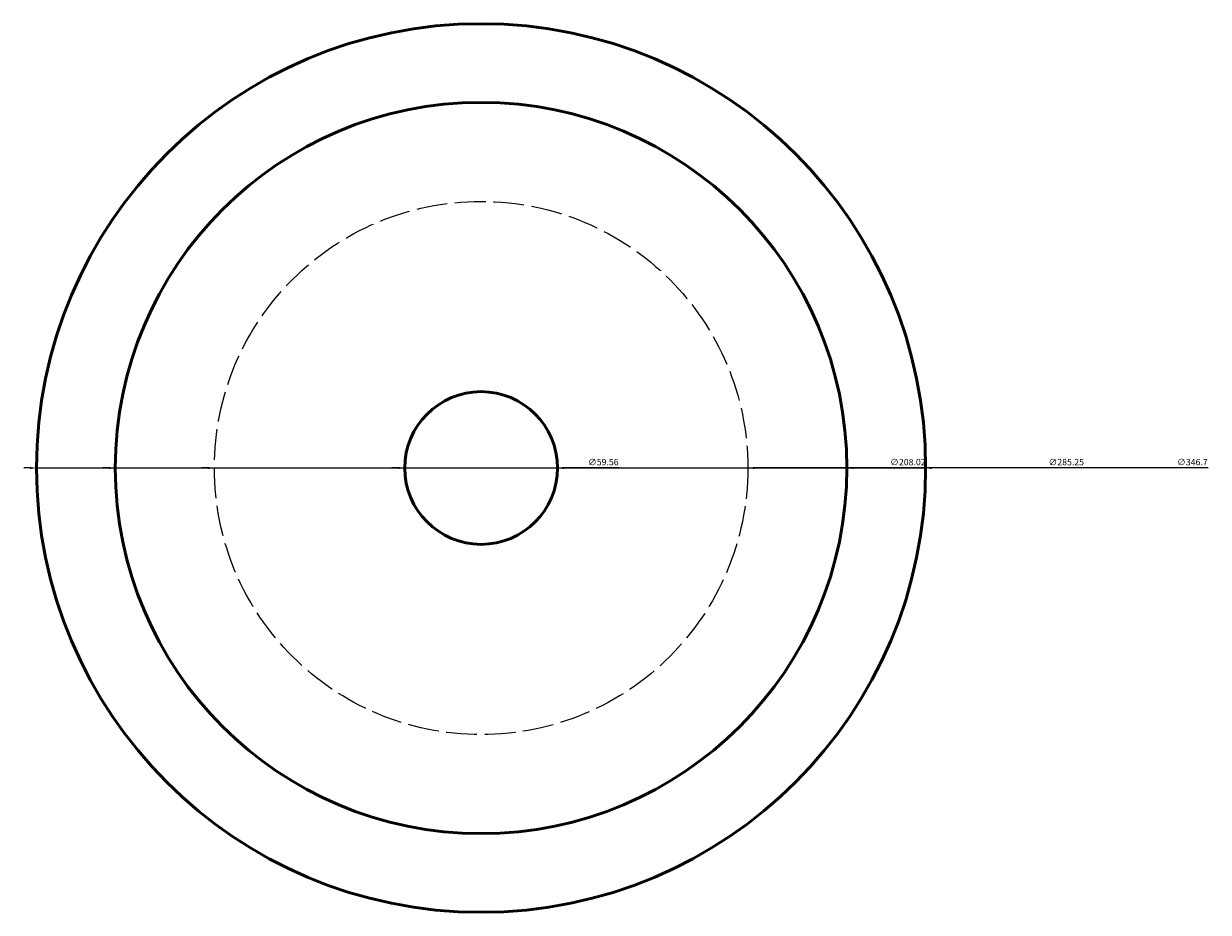
# Model space of a CAD drawing. Units: millimetres. Extents: x 921 to 2648, y 1390 to 2315.
# Tile 10 of 10: x 1802 to 2264, y 1968 to 2315. Entities that reach past the tile are written whole.
import ezdxf

# ---------------------------------------------------------------- set-up
doc = ezdxf.new("R2010")
doc.units = ezdxf.units.MM
doc.linetypes.add('ACAD_ISO02W100', pattern=[15, 12, -3])
for name, color, linetype, lineweight in [('M-DIMS', 2, 'Continuous', 25), ('M-HIDN', 4, 'ACAD_ISO02W100', 25), ('M-OUTL', 7, 'Continuous', 50)]:
    doc.layers.add(name, color=color, linetype=linetype, lineweight=lineweight)
doc.styles.get("Standard").update_dxf_attribs({"font": 'arial.ttf'})
doc.dimstyles.new('ISO-25', dxfattribs={"dimtxt": 2.5, "dimasz": 2.5, "dimexe": 1.25, "dimexo": 0.625, "dimtad": 1, "dimtxsty": 'Standard', "dimcen": 2.5, "dimadec": 0, "dimazin": 0, "dimtfac": 1, "dimtmove": 0, "dimatfit": 3, "dimfxl": 1, "dimarcsym": 0})

# ---------------------------------------------------------------- blocks, each defined once
blk = doc.blocks.new('*D102')
at = {"layer": 'Defpoints', "color": 0, "transparency": 16777216}
for p in [(1806.98, 2141.54), (2153.69, 2141.54)]:
    blk.add_point(p, dxfattribs=at)
at = {"layer": 'M-DIMS', "color": 0, "lineweight": -2, "transparency": 16777216}
for p, q in [((1804.48, 2141.54), (1801.98, 2141.54)), ((1806.98, 2141.54), (2153.69, 2141.54)), ((2263.91, 2141.54), (2156.19, 2141.54))]:
    blk.add_line(p, q, dxfattribs=at)
at = {"layer": 'M-DIMS', "color": 0, "transparency": 16777216}
for points in [[(1804.48, 2141.95), (1804.48, 2141.12), (1806.98, 2141.54)], [(2156.19, 2141.95), (2156.19, 2141.12), (2153.69, 2141.54)]]:
    blk.add_solid(points, dxfattribs=at)
at = {"layer": 'M-DIMS', "color": 0, "transparency": 16777216, "insert": (2257.7, 2143.51), "char_height": 2.5, "attachment_point": 5, "rotation": 360}
blk.add_mtext('∅346.7', dxfattribs=at)
blk = doc.blocks.new('*D103')
at = {"layer": 'Defpoints', "color": 0, "transparency": 16777216}
for p in [(1837.71, 2141.54), (2122.96, 2141.54)]:
    blk.add_point(p, dxfattribs=at)
at = {"layer": 'M-DIMS', "color": 0, "lineweight": -2, "transparency": 16777216}
for p, q in [((1835.21, 2141.54), (1832.71, 2141.54)), ((1837.71, 2141.54), (2122.96, 2141.54)), ((2215.72, 2141.54), (2125.46, 2141.54))]:
    blk.add_line(p, q, dxfattribs=at)
at = {"layer": 'M-DIMS', "color": 0, "transparency": 16777216}
for points in [[(1835.21, 2141.95), (1835.21, 2141.12), (1837.71, 2141.54)], [(2125.46, 2141.95), (2125.46, 2141.12), (2122.96, 2141.54)]]:
    blk.add_solid(points, dxfattribs=at)
at = {"layer": 'M-DIMS', "color": 0, "transparency": 16777216, "insert": (2208.53, 2143.51), "char_height": 2.5, "attachment_point": 5, "rotation": 360}
blk.add_mtext('∅285.25', dxfattribs=at)
blk = doc.blocks.new('*D104')
at = {"layer": 'Defpoints', "color": 0, "transparency": 16777216}
for p in [(1876.32, 2141.54), (2084.35, 2141.54)]:
    blk.add_point(p, dxfattribs=at)
at = {"layer": 'M-DIMS', "color": 0, "lineweight": -2, "transparency": 16777216}
for p, q in [((1873.82, 2141.54), (1871.32, 2141.54)), ((1876.32, 2141.54), (2084.35, 2141.54)), ((2153.92, 2141.54), (2086.85, 2141.54))]:
    blk.add_line(p, q, dxfattribs=at)
at = {"layer": 'M-DIMS', "color": 0, "transparency": 16777216}
for points in [[(1873.82, 2141.95), (1873.82, 2141.12), (1876.32, 2141.54)], [(2086.85, 2141.95), (2086.85, 2141.12), (2084.35, 2141.54)]]:
    blk.add_solid(points, dxfattribs=at)
at = {"layer": 'M-DIMS', "color": 0, "transparency": 16777216, "insert": (2146.76, 2143.51), "char_height": 2.5, "attachment_point": 5, "rotation": 360}
blk.add_mtext('∅208.02', dxfattribs=at)
blk = doc.blocks.new('*D105')
at = {"layer": 'Defpoints', "color": 0, "transparency": 16777216}
for p in [(1950.55, 2141.54), (2010.12, 2141.54)]:
    blk.add_point(p, dxfattribs=at)
at = {"layer": 'M-DIMS', "color": 0, "lineweight": -2, "transparency": 16777216}
for p, q in [((1948.05, 2141.54), (1945.55, 2141.54)), ((1950.55, 2141.54), (2010.12, 2141.54)), ((2034.19, 2141.54), (2012.62, 2141.54))]:
    blk.add_line(p, q, dxfattribs=at)
at = {"layer": 'M-DIMS', "color": 0, "transparency": 16777216}
for points in [[(1948.05, 2141.95), (1948.05, 2141.12), (1950.55, 2141.54)], [(2012.62, 2141.95), (2012.62, 2141.12), (2010.12, 2141.54)]]:
    blk.add_solid(points, dxfattribs=at)
at = {"layer": 'M-DIMS', "color": 0, "transparency": 16777216, "insert": (2027.99, 2143.51), "char_height": 2.5, "attachment_point": 5, "rotation": 359.9999}
blk.add_mtext('∅59.56', dxfattribs=at)

msp = doc.modelspace()

# ---------------------------------------------------------------- linework, layer by layer
at = {"layer": 'M-HIDN'}
msp.add_circle((1980.3371, 2141.536), 104.0122, dxfattribs=at)
at = {"layer": 'M-OUTL'}
for radius in [173.3537, 142.6229, 29.7824]:
    msp.add_circle((1980.3371, 2141.536), radius, dxfattribs=at)

# ---------------------------------------------------------------- dimensions: what is measured, and where the dimension line sits
at = {"layer": 'M-DIMS'}
for p1, p2, override, picture, middle in [((1806.9834, 2141.5361), (2153.6909, 2141.536), {"dimdec": 1, "dimlfac": 1, "dimrnd": 0, "dimzin": 0, "dimdsep": 46, "dimlunit": 2}, '*D102', (2257.7031, 2141.536)), ((1837.7143, 2141.5361), (2122.96, 2141.536), {"dimdec": 2, "dimlfac": 1, "dimrnd": 0, "dimzin": 0, "dimdsep": 46, "dimlunit": 2}, '*D103', (2208.5337, 2141.536)), ((1876.3249, 2141.5361), (2084.3494, 2141.536), {"dimdec": 2, "dimlfac": 1, "dimrnd": 0, "dimzin": 0, "dimdsep": 46, "dimlunit": 2}, '*D104', (2146.7567, 2141.536)), ((1950.5547, 2141.5361), (2010.1196, 2141.536), {"dimdec": 2, "dimlfac": 1, "dimrnd": 0, "dimzin": 0, "dimdsep": 46, "dimlunit": 2}, '*D105', (2027.989, 2141.536))]:
    dim = msp.add_diameter_dim_2p(p1=p1, p2=p2, dimstyle='ISO-25', override=override, dxfattribs=at)
    dim.commit()
    dim.dimension.update_dxf_attribs({"geometry": picture, "text_midpoint": middle, "dimtype": 163})

doc.saveas('drawing.dxf')
